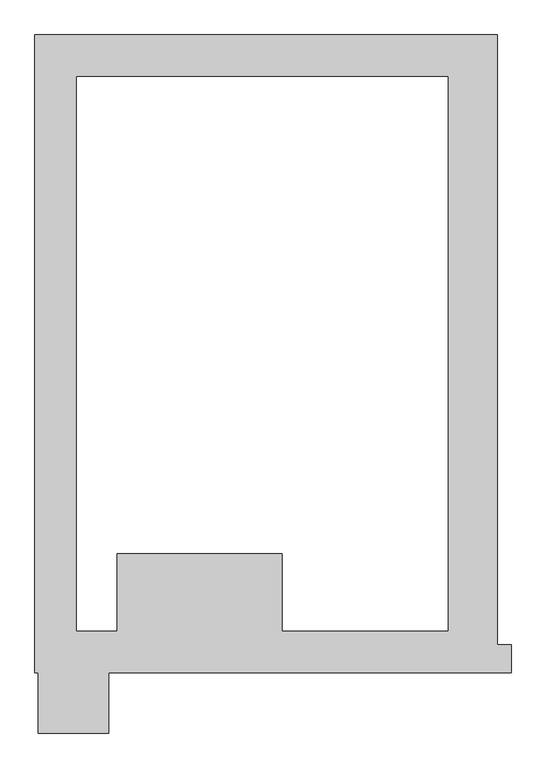
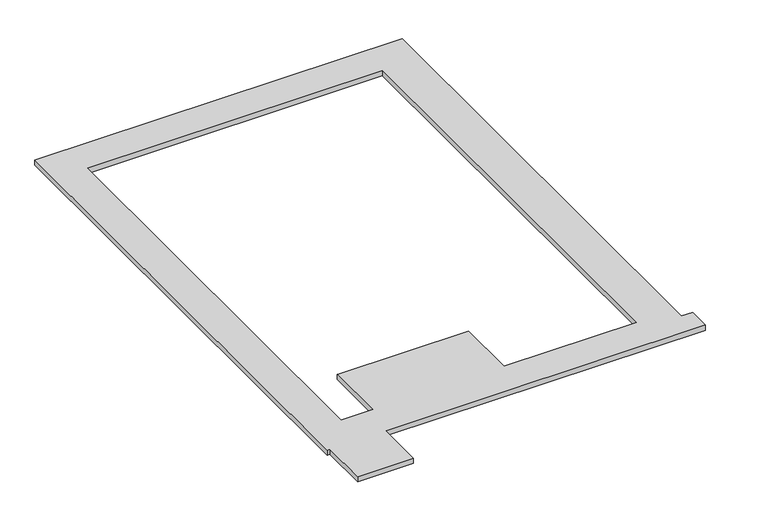
"""IFC4 building model written with IfcOpenShell, lengths in millimetres: proxy geometry."""

from ifc_helpers import new_model, si_unit, frame, origin, place, context, project, spatial, polyline, outline, extrude, source, transform, mapped, element, save


def roads_a759df18(model_context):
    return source(origin(), model_context, "Body", "SweptSolid", [
        extrude(outline(polyline([(-25562.3656867, -6179.7520828), (-25562.3656867, 7688.6479172), (-15503.9656867, 7688.6479172), (-15503.9656867, -5570.1520828), (-15199.1656867, -5570.1520828), (-15199.1656867, -6179.7520828), (-23962.1656867, -6179.7520828), (-23962.1656867, -7491.5257947), (-25486.1656867, -7491.5257947), (-25486.1656867, -6179.7520828), (-25562.3656867, -6179.7520828)]), holes=[polyline([(-24647.9656867, 6774.2479172), (-24647.9656867, -5265.3520828), (-23785.8963079, -5265.3520828), (-23785.8963079, -3579.9257947), (-20179.0963079, -3579.9257947), (-20179.0963079, -5265.3520828), (-16570.7656867, -5265.3520828), (-16570.7656867, 6774.2479172), (-24647.9656867, 6774.2479172)])]), frame((0.0, 0.0, -1981.2), z_axis=(0.0, 0.0, 1.0), x_axis=(1.0, 0.0, 0.0)), (0.0, 0.0, 1.0), 152.4),
    ])


if __name__ == "__main__":
    model = new_model("IFC4")
    model_context = context("Model", 3, world=origin())
    ifc_project = project(units=[si_unit("LENGTHUNIT", "METRE", prefix="MILLI")], contexts=[model_context])
    site = spatial("IfcSite", under=ifc_project)
    building = spatial("IfcBuilding", under=site)
    placement = place(None, origin())
    roads_shape = roads_a759df18(model_context)
    element("IfcBuildingElementProxy", 1, Name="Roads", at=placement, inside=building, context=model_context, shape_type="MappedRepresentation", body=[
        mapped(roads_shape, transform((0.0, 0.0, 0.0), x_axis=(1.0, 0.0, 0.0), y_axis=(0.0, 1.0, 0.0), z_axis=(0.0, 0.0, 1.0))),
    ])
    save(model, "model.ifc")

# Revit data of these elements
# Element 1 (IfcBuildingElementProxy)
#   Materials on its faces: "Damp-proofing"
# Materials
#   "Damp-proofing": class "Generic", colour RGB 17 17 17, transparency 0, Description = "Damp-proofing", Cost = 0
